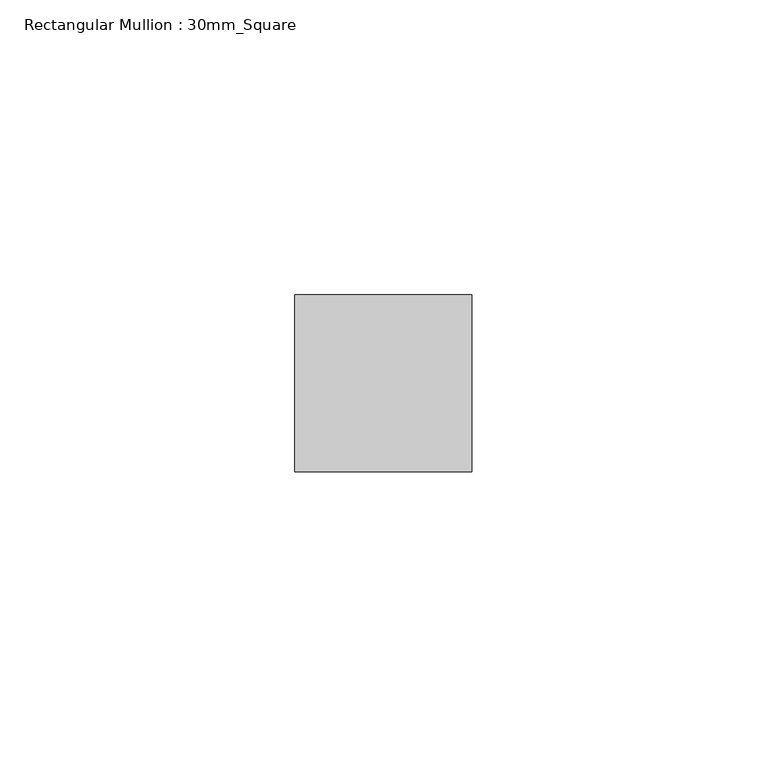
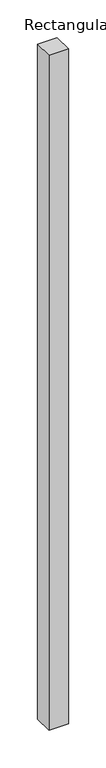
"""IFC4 building model written with IfcOpenShell, lengths in millimetres: member geometry, Rectangular Mullion : 30mm_Square."""

from ifc_helpers import new_model, si_unit, frame, origin, place, context, project, spatial, polyline, outline, extrude, source, transform, mapped, element, save


def rectangular_mullion_30mm_square_eec092c3(model_context):
    return source(origin(), model_context, "Body", "SweptSolid", [
        extrude(outline(polyline([(0.0, 15.0), (0.0, -15.0), (-30.0, -15.0), (-30.0, 15.0), (0.0, 15.0)])), frame((0.0, 0.0, -1092.6063046), z_axis=(0.0, 0.0, 1.0), x_axis=(1.0, 0.0, 0.0)), (0.0, 0.0, 1.0), 1092.6063046),
    ])


if __name__ == "__main__":
    model = new_model("IFC4")
    model_context = context("Model", 3, world=origin())
    ifc_project = project(units=[si_unit("LENGTHUNIT", "METRE", prefix="MILLI")], contexts=[model_context])
    site = spatial("IfcSite", under=ifc_project)
    building = spatial("IfcBuilding", under=site)
    placement = place(None, origin())
    rectangular_mullion_30mm_square_shape = rectangular_mullion_30mm_square_eec092c3(model_context)
    element("IfcMember", 1, ObjectType="Rectangular Mullion : 30mm_Square", at=placement, inside=building, context=model_context, shape_type="MappedRepresentation", body=[
        mapped(rectangular_mullion_30mm_square_shape, transform((0.0, 0.0, 0.0), x_axis=(1.0, 0.0, 0.0), y_axis=(0.0, 1.0, 0.0), z_axis=(0.0, 0.0, 1.0))),
    ])
    save(model, "model.ifc")

# Revit data of these elements
# Type "Rectangular Mullion : 30mm_Square"
#   Keynote = "H11"
#   built-in parameter 1007304 = 0.0984252 (stored number, unit not read)
#   built-in parameter 1007301 = 0.0492126 (stored number, unit not read)
#   built-in parameter 1007300 = 0.0492126 (stored number, unit not read)
# Element 1 (IfcMember, "Rectangular Mullion : 30mm_Square")
#   Materials on its faces: "Aluminium"
# Materials
#   "Aluminium": class "Metal", colour RGB 247 247 247, transparency 0, Description = "Aluminium 6061", Cost = 0
